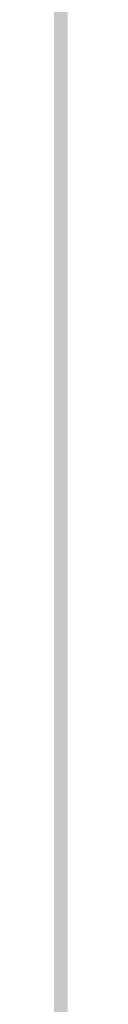
# Model space of a CAD drawing. Units: inches. Extents: x 2083 to 3317, y 1141 to 2115.
# Tile 175 of 256: x 3126.95969 to 3126.95976, y 1263.27402 to 1263.29018. Entities that reach past the tile are written whole.
import ezdxf

# ---------------------------------------------------------------- set-up
doc = ezdxf.new("R2010")
doc.units = ezdxf.units.IN
doc.layers.add('A-ANNO-DIMS', color=2, linetype='Continuous', lineweight=18)
doc.layers.add('A-WALL-PATT', color=251, linetype='Continuous', lineweight=13, true_color=0x636466)
doc.styles.get("Standard").update_dxf_attribs({"font": 'arial.ttf'})
doc.dimstyles.new('ISO-25', dxfattribs={"dimtxt": 12, "dimasz": 12, "dimexe": 1.25, "dimexo": 0.625, "dimtad": 1, "dimlunit": 3, "dimtxsty": 'Standard', "dimcen": 2.5, "dimadec": 0, "dimazin": 0, "dimtfac": 1, "dimtmove": 0, "dimatfit": 3, "dimfxl": 1, "dimarcsym": 0})

# ---------------------------------------------------------------- blocks, each defined once
blk = doc.blocks.new('*D26')
at = {"layer": 'A-ANNO-DIMS', "color": 0, "lineweight": -2, "transparency": 16777216}
for p, q in [((3088.985844, 1274.915092), (3088.985844, 1270.951963)), ((3111.240037, 1274.915092), (3111.240037, 1270.951963)), ((3076.985844, 1272.201963), (2840.262447, 1272.201963)), ((3111.240037, 1272.201963), (3088.985844, 1272.201963)), ((3123.240037, 1272.201963), (3135.240037, 1272.201963))]:
    blk.add_line(p, q, dxfattribs=at)
at = {"layer": 'A-ANNO-DIMS', "color": 0, "transparency": 16777216}
for points in [[(3076.985844, 1274.201963), (3076.985844, 1270.201963), (3088.985844, 1272.201963)], [(3123.240037, 1274.201963), (3123.240037, 1270.201963), (3111.240037, 1272.201963)]]:
    blk.add_solid(points, dxfattribs=at)
at = {"layer": 'Defpoints', "color": 0, "transparency": 16777216}
for p in [(3088.985844, 1275.540092), (3111.240037, 1275.540092), (3088.985844, 1272.201963)]:
    blk.add_point(p, dxfattribs=at)
at = {"layer": 'A-ANNO-DIMS', "color": 0, "transparency": 16777216, "insert": (2952.624146, 1279.031602), "char_height": 12, "attachment_point": 5}
blk.add_mtext('NIGHTSTAND 1\'-10 1/2" TYP.', dxfattribs=at)
blk = doc.blocks.new('*D27')
at = {"layer": 'A-ANNO-DIMS', "color": 0, "lineweight": -2, "transparency": 16777216}
for p, q in [((3114.578165, 1309.794285), (3114.578165, 1321.794285)), ((3111.865037, 1297.794285), (3115.828165, 1297.794285)), ((3114.578165, 1297.794285), (3114.578165, 1275.540092)), ((3111.865037, 1275.540092), (3115.828165, 1275.540092)), ((3114.578165, 1263.540092), (3114.578165, 1140.988591))]:
    blk.add_line(p, q, dxfattribs=at)
at = {"layer": 'A-ANNO-DIMS', "color": 0, "transparency": 16777216}
for points in [[(3112.578165, 1309.794285), (3116.578165, 1309.794285), (3114.578165, 1297.794285)], [(3112.578165, 1263.540092), (3116.578165, 1263.540092), (3114.578165, 1275.540092)]]:
    blk.add_solid(points, dxfattribs=at)
at = {"layer": 'Defpoints', "color": 0, "transparency": 16777216}
for p in [(3111.240037, 1297.794285), (3111.240037, 1275.540092), (3114.578165, 1275.540092)]:
    blk.add_point(p, dxfattribs=at)
at = {"layer": 'A-ANNO-DIMS', "color": 0, "transparency": 16777216, "insert": (3107.748527, 1196.264342), "char_height": 12, "attachment_point": 5, "rotation": 90}
blk.add_mtext('1\'-10 1/2" TYP.', dxfattribs=at)

msp = doc.modelspace()

# ---------------------------------------------------------------- hatches: boundary and pattern name
at = {"layer": 'A-WALL-PATT'}
h = msp.add_hatch(color=256, dxfattribs=at)
h.dxf.hatch_style = 1
h.paths.add_polyline_path([(3126.959783, 2020.76136), (2748.959783, 2020.76136), (2604.959783, 2020.76136), (2226.959783, 2020.76136), (2226.959783, 1702.76136), (2466.959783, 1702.76136), (2466.959783, 1582.76136), (2418.959783, 1582.76136), (2418.959783, 1477.76136), (2226.959783, 1477.76136), (2226.959783, 1263.26136), (2544.959783, 1263.26136), (2544.959783, 1411.76136), (2604.959783, 1411.76136), (2685.959783, 1411.76136), (2685.959783, 1420.76136), (2604.959783, 1420.76136), (2604.959783, 1573.76136), (2604.959783, 1702.76136), (2604.959783, 2011.76136), (2748.959783, 2011.76136), (2748.959783, 1702.76136), (2862.959783, 1702.76136), (2862.959783, 1621.76136), (2871.959783, 1621.76136), (2871.959783, 1702.76136), (2883.959783, 1702.76136), (2883.959783, 1706.939459, -0.026459), (2883.959783, 1711.76136), (2757.959783, 1711.76136), (2757.959783, 1807.76136), (2787.959783, 1807.76136), (2787.959783, 1812.26136), (2757.959783, 1812.26136), (2757.959783, 2011.76136), (2877.959783, 2011.76136), (2877.959783, 1812.26136), (2847.959783, 1812.26136), (2847.959783, 1807.76136), (2889.835742, 1807.76136), (2889.835742, 1812.26136), (2882.459783, 1812.26136), (2882.459783, 2011.76136), (3117.959783, 2011.76136), (3117.959783, 1812.26136), (2937.835742, 1812.26136), (2937.835742, 1807.76136), (2995.709783, 1807.76136), (2995.709783, 1796.117666), (3000.209783, 1796.117666), (3000.209783, 1807.76136), (3117.959783, 1807.76136), (3117.959783, 1711.76136), (3000.209783, 1711.76136), (3000.209783, 1760.117666), (2998.572705, 1760.117666, -0.020711), (2995.709783, 1760.117666), (2995.709783, 1711.76136), (2931.959783, 1711.76136), (2931.959783, 1702.76136), (3126.959783, 1702.76136)])
h.paths.add_polyline_path([(2471.459783, 2011.76136), (2471.459783, 1810.01136), (2462.716936, 1810.01136), (2462.716936, 1805.51136), (2505.959783, 1805.51136), (2505.959783, 1810.01136), (2475.959783, 1810.01136), (2475.959783, 2011.76136), (2595.959783, 2011.76136), (2595.959783, 1810.01136), (2565.959783, 1810.01136), (2565.959783, 1805.51136), (2595.959783, 1805.51136), (2595.959783, 1711.76136), (2235.959783, 1711.76136), (2235.959783, 1805.51136), (2353.709783, 1805.51136), (2353.709783, 1796.054162), (2358.209783, 1796.054162), (2358.209783, 1805.51136), (2414.716936, 1805.51136), (2414.716936, 1810.01136), (2235.959783, 1810.01136), (2235.959783, 2011.76136)], flags=16)
h.paths.add_polyline_path([(2270.204734, 1994.610008), (2270.204734, 1970.610008), (2246.204734, 1970.610008), (2246.204734, 1994.610008)], flags=0)
edge = h.paths.add_edge_path(flags=0)
edge.add_ellipse((2332.027391, 1899.798176), major_axis=(-3.042994, 3.042994), ratio=0.16825245, start_angle=-161.332166, end_angle=-156.307114, ccw=False)
edge.add_ellipse((2333.082037, 1898.74353), major_axis=(-1.054646, 1.054646), ratio=0.4535321, start_angle=-123.371019, end_angle=-94.159107)
edge = h.paths.add_edge_path(flags=0)
edge.add_ellipse((2332.027391, 1968.87629), major_axis=(3.042994, 3.042994), ratio=0.16825245, start_angle=18.667834, end_angle=23.692886)
edge.add_spline(control_points=[(2332.925596, 1970.691105), (2332.226768, 1970.3361), (2330.893709, 1969.658905), (2328.41308, 1970.932138), (2327.203934, 1967.748712), (2324.709596, 1969.955589), (2322.532822, 1967.012354), (2320.012846, 1971.295812), (2317.680308, 1968.157845), (2316.040526, 1967.102047), (2315.426904, 1966.809602)], knot_values=[0, 0, 0, 0, 2.267059, 4.324559, 6.685584, 8.878641, 11.121502, 14.300359, 17.755284, 19.732645, 19.732645, 19.732645, 19.732645], degree=3, periodic=0)
edge.add_ellipse((2332.027391, 1968.87629), major_axis=(3.042994, 3.042994), ratio=0.16825245, start_angle=18.667834, end_angle=23.692886, ccw=False)
edge.add_ellipse((2333.082037, 1969.930936), major_axis=(1.054646, 1.054646), ratio=0.4535321, start_angle=56.628981, end_angle=85.840893, ccw=False)
edge = h.paths.add_edge_path(flags=0)
edge.add_spline(control_points=[(2296.428287, 1967.987908), (2293.627804, 1965.336314), (2287.703624, 1959.727094), (2299.74386, 1949.995699), (2294.532591, 1935.668528), (2290.573228, 1920.603512), (2293.394124, 1909.973691), (2296.185407, 1904.966543)], knot_values=[0.099185, 0.099185, 0.099185, 0.099185, 0.345301, 0.619822, 0.982653, 1.386093, 1.810555, 1.810555, 1.810555, 1.810555], degree=3, periodic=0)
edge.add_spline(control_points=[(2296.185407, 1904.966543), (2297.383582, 1902.6193), (2298.000969, 1901.949312), (2298.55297, 1901.468155)], knot_values=[0.006246, 0.006246, 0.006246, 0.006246, 0.055476, 0.055476, 0.055476, 0.055476], degree=3, periodic=0)
edge.add_spline(control_points=[(2298.55297, 1901.468155), (2297.258612, 1900.923224), (2295.225294, 1900.232126), (2293.060229, 1900.614205), (2292.101423, 1900.788415), (2292.089578, 1900.790568)], knot_values=[0.312835, 0.312835, 0.312835, 0.312835, 0.40178, 0.474987, 0.475903, 0.475903, 0.475903, 0.475903], degree=3, periodic=0)
edge.add_arc((2292.793646, 1904.664109), 3.937008, 215.420897, 259.698179, ccw=False)
edge.add_spline(control_points=[(2289.585314, 1902.382304), (2289.476652, 1902.535087), (2289.36848, 1902.688035), (2289.260865, 1902.84117)], knot_values=[0.102872, 0.102872, 0.102872, 0.102872, 0.116896, 0.116896, 0.116896, 0.116896], degree=3, periodic=0)
edge.add_spline(control_points=[(2289.260865, 1902.84117), (2288.686604, 1902.550192), (2287.640048, 1902.019902), (2285.881337, 1901.873954), (2283.852972, 1901.504352), (2281.719987, 1899.710538), (2278.466991, 1899.492942), (2276.157136, 1901.883202), (2272.258953, 1899.804071), (2267.777605, 1901.843183), (2262.243882, 1900.184033), (2257.414927, 1901.782061), (2254.318374, 1900.72612), (2253.178285, 1900.337343)], knot_values=[0, 0, 0, 0, 1.907977, 3.477176, 5.261074, 7.972851, 11.680248, 13.717921, 16.939592, 22.789562, 27.502503, 33.595215, 37.145618, 37.145618, 37.145618, 37.145618], degree=3, periodic=0)
edge.add_line((2253.178285, 1900.337343), (2250.24424, 1902.84117))
edge.add_line((2250.24424, 1902.84117), (2250.24424, 1965.833296))
edge.add_line((2250.24424, 1965.833296), (2253.178285, 1968.337123))
edge.add_spline(control_points=[(2253.178285, 1968.337123), (2254.318374, 1967.948346), (2257.414927, 1966.892405), (2262.243882, 1968.490433), (2267.777605, 1966.831283), (2271.52673, 1968.537217), (2273.875914, 1967.828289), (2274.206701, 1967.727642)], knot_values=[0, 0, 0, 0, 0.09018, 0.244935, 0.364644, 0.513233, 0.537855, 0.537855, 0.537855, 0.537855], degree=3, periodic=0)
edge.add_arc((2274.352887, 1963.793349), 3.937008, 72.051134, 92.127949, ccw=False)
edge.add_arc((2281.296933, 1985.230003), 18.596298, 252.0511336, 288.5657217)
edge.add_arc((2292.316717, 1956.02888), 12.646081, 71.0267879, 113.7782184, ccw=False)
edge = h.paths.add_edge_path(flags=0)
edge.add_spline(control_points=[(2274.899415, 1951.856195), (2275.066156, 1951.616592), (2275.232687, 1951.376588), (2275.397987, 1951.135855)], knot_values=[1.409916, 1.409916, 1.409916, 1.409916, 1.43159, 1.43159, 1.43159, 1.43159], degree=3, periodic=0)
edge.add_spline(control_points=[(2275.397987, 1951.135855), (2275.792106, 1950.561885), (2276.179231, 1949.983774), (2276.545546, 1949.397103)], knot_values=[1.358238, 1.358238, 1.358238, 1.358238, 1.409916, 1.409916, 1.409916, 1.409916], degree=3, periodic=0)
edge.add_line((2276.545546, 1949.397103), (2277.437289, 1947.862185))
edge.add_spline(control_points=[(2277.437289, 1947.862185), (2276.303834, 1945.673115), (2274.639698, 1942.426882), (2274.631615, 1938.0939), (2272.799124, 1930.85155), (2274.356426, 1943.897046), (2275.947681, 1947.923356), (2276.545546, 1949.397103)], knot_values=[0.005632, 0.005632, 0.005632, 0.005632, 0.186014, 0.266002, 0.357087, 0.59639, 0.739732, 0.739732, 0.739732, 0.739732], degree=3, periodic=0)
edge.add_spline(control_points=[(2276.545546, 1949.397103), (2276.179231, 1949.983774), (2275.792106, 1950.561885), (2275.397987, 1951.135855)], knot_values=[1.358238, 1.358238, 1.358238, 1.358238, 1.409916, 1.409916, 1.409916, 1.409916], degree=3, periodic=0)
edge.add_spline(control_points=[(2275.397987, 1951.135855), (2274.9425, 1950.080452), (2274.20776, 1948.025272), (2273.934602, 1944.851477), (2272.468534, 1937.627489), (2273.466216, 1945.696466), (2274.700615, 1951.059472), (2274.899415, 1951.856195)], knot_values=[0.104364, 0.104364, 0.104364, 0.104364, 0.189636, 0.269624, 0.36071, 0.600013, 0.644622, 0.644622, 0.644622, 0.644622], degree=3, periodic=0)
h.paths.add_polyline_path([(2269.167514, 1963.127573, -0.357527), (2268.170633, 1960.97637, -0.092561), (2268.170633, 1939.436325, -0.357527), (2269.167514, 1937.285122, -0.357527), (2267.01631, 1938.282002, -0.164785), (2254.685581, 1938.282002, -0.357527), (2252.534378, 1937.285122, -0.357527), (2253.531259, 1939.436325, -0.092561), (2253.531259, 1960.97637, -0.357527), (2252.534378, 1963.127573, -0.357527), (2254.685581, 1962.130692, -0.164785), (2267.01631, 1962.130692, -0.357527)], flags=0)
h.paths.add_polyline_path([(2248.874068, 1967.8018), (2248.874068, 1957.02771), (2249.457783, 1957.02771), (2249.457783, 1911.646756), (2248.874068, 1911.646756), (2248.874068, 1900.872666), (2246.511863, 1900.872666, 0.197327), (2244.149658, 1902.456873), (2244.149658, 1966.217592, 0.197327), (2246.511863, 1967.8018)], flags=0)
h.paths.add_polyline_path([(2269.167514, 1931.389344, -0.357527), (2268.170633, 1929.238141, -0.092561), (2268.170633, 1907.698096, -0.357527), (2269.167514, 1905.546893, -0.357527), (2267.01631, 1906.543774, -0.164785), (2254.685581, 1906.543774, -0.357527), (2252.534378, 1905.546893, -0.357527), (2253.531259, 1907.698096, -0.092561), (2253.531259, 1929.238141, -0.357527), (2252.534378, 1931.389344, -0.357527), (2254.685581, 1930.392463, -0.164785), (2267.01631, 1930.392463, -0.357527)], flags=0)
edge = h.paths.add_edge_path(flags=0)
edge.add_spline(control_points=[(2276.196858, 1906.723702), (2276.168144, 1909.028928), (2276.114049, 1913.371852), (2270.598417, 1924.924978), (2273.905175, 1919.012779), (2275.921711, 1916.262063), (2275.47457, 1912.402149), (2277.257874, 1910.380621), (2276.696044, 1908.225036), (2276.646218, 1906.813023), (2276.617825, 1906.008407)], knot_values=[0, 0, 0, 0, 8.61026, 16.221274, 18.843057, 23.804898, 27.440828, 29.356102, 31.203478, 33.650687, 33.650687, 33.650687, 33.650687], degree=3, periodic=0)
edge.add_spline(control_points=[(2276.617825, 1906.008407), (2276.623313, 1905.624144), (2276.497738, 1904.628661), (2275.441779, 1903.854725), (2274.937314, 1903.08045), (2274.85908, 1902.84117)], knot_values=[0.156488, 0.156488, 0.156488, 0.156488, 0.184398, 0.231376, 0.250598, 0.250598, 0.250598, 0.250598], degree=3, periodic=0)
edge.add_line((2274.85908, 1902.84117), (2276.50598, 1902.84117))
edge.add_spline(control_points=[(2276.50598, 1902.84117), (2276.788308, 1903.08494), (2277.665071, 1904.125196), (2278.249538, 1904.340738), (2277.653872, 1908.527387), (2278.15567, 1906.227808), (2278.100464, 1905.285948), (2278.846675, 1904.069005), (2277.856785, 1903.414948), (2277.874191, 1902.99105), (2277.903562, 1902.84117)], knot_values=[0.059574, 0.059574, 0.059574, 0.059574, 0.080753, 0.103741, 0.16972, 0.176036, 0.207137, 0.240474, 0.262341, 0.27366, 0.27366, 0.27366, 0.27366], degree=3, periodic=0)
edge.add_line((2277.903562, 1902.84117), (2280.029825, 1902.84117))
edge.add_spline(control_points=[(2280.029825, 1902.84117), (2279.888221, 1903.088398), (2279.499257, 1903.981551), (2280.152284, 1905.939349), (2278.103615, 1909.657757), (2279.762395, 1907.185285), (2280.3279, 1904.874861), (2280.485109, 1903.48959), (2281.463269, 1903.249432), (2281.758343, 1902.936497), (2281.834036, 1902.84117)], knot_values=[0.013856, 0.013856, 0.013856, 0.013856, 0.034874, 0.088867, 0.107879, 0.126738, 0.158714, 0.193757, 0.217487, 0.226722, 0.226722, 0.226722, 0.226722], degree=3, periodic=0)
edge.add_spline(control_points=[(2281.834036, 1902.84117), (2281.787535, 1902.826703), (2281.647022, 1902.782988), (2281.395527, 1902.85949), (2281.088077, 1902.985242), (2280.720683, 1903.060902), (2280.333451, 1903.025726), (2280.124767, 1902.898879), (2280.029825, 1902.84117)], knot_values=[0, 0, 0, 0, 0.14413, 0.435517, 0.749276, 1.153046, 1.548371, 1.878348, 1.878348, 1.878348, 1.878348], degree=3, periodic=0)
edge.add_line((2280.029825, 1902.84117), (2277.903562, 1902.84117))
edge.add_spline(control_points=[(2277.903562, 1902.84117), (2277.892855, 1902.795855), (2277.865396, 1902.679637), (2277.607479, 1902.687483), (2277.27405, 1902.8007), (2276.837921, 1902.619775), (2276.583807, 1902.789261), (2276.50598, 1902.84117)], knot_values=[0, 0, 0, 0, 0.127189, 0.326199, 0.628009, 1.24357, 1.515331, 1.515331, 1.515331, 1.515331], degree=3, periodic=0)
edge.add_line((2276.50598, 1902.84117), (2274.85908, 1902.84117))
edge.add_spline(control_points=[(2274.85908, 1902.84117), (2274.814437, 1902.898587), (2274.72513, 1903.013446), (2274.493477, 1903.118968), (2274.244285, 1902.960539), (2273.937121, 1903.184942), (2273.614039, 1902.983143), (2273.408316, 1902.883045), (2273.322254, 1902.84117)], knot_values=[0, 0, 0, 0, 0.21843, 0.436957, 0.687977, 0.990379, 1.398396, 1.69185, 1.69185, 1.69185, 1.69185], degree=3, periodic=0)
edge.add_spline(control_points=[(2273.322254, 1902.84117), (2273.61674, 1903.445692), (2274.273998, 1904.538253), (2276.027239, 1904.573702), (2276.206963, 1906.583637), (2276.196858, 1906.723702)], knot_values=[0.012227, 0.012227, 0.012227, 0.012227, 0.059472, 0.106218, 0.134458, 0.134458, 0.134458, 0.134458], degree=3, periodic=0)
h.paths.add_polyline_path([(2270.776054, 1897.789828), (2270.776054, 1873.789828), (2246.776054, 1873.789828), (2246.776054, 1897.789828)], flags=0)
h.paths.add_polyline_path([(2353.709783, 1760.005059), (2353.709783, 1760.054162), (2358.209783, 1760.054162, -0.033729)], flags=0)
h.paths.add_polyline_path([(2321.819119, 1737.529186), (2341.995327, 1737.529186, -0.414214), (2343.203273, 1736.321241), (2343.203273, 1721.020596, -0.414214), (2341.995327, 1719.812651), (2321.819119, 1719.812651, -0.414214), (2320.611173, 1721.020596), (2320.611173, 1736.321241, -0.414214)], flags=0)
h.paths.add_polyline_path([(2324.23501, 1736.321241), (2339.579436, 1736.321241, -0.414214), (2341.995327, 1733.905349), (2341.995327, 1725.44973, -0.414214), (2339.579436, 1723.033839), (2333.680588, 1723.033839), (2333.845317, 1722.045467, -0.870646), (2335.425399, 1721.825893, -0.767327), (2333.922694, 1721.423245), (2331.291024, 1721.423245, -0.767327), (2329.788319, 1721.825893, -0.870646), (2331.368401, 1722.045467), (2331.53313, 1723.033839), (2324.23501, 1723.033839, -0.414214), (2321.819119, 1725.44973), (2321.819119, 1733.905349, -0.414214)], flags=0)
h.paths.add_polyline_path([(2570.483789, 1928.615444), (2589.683789, 1928.615444), (2590.168829, 1928.615444), (2590.168829, 1904.993397), (2570.483789, 1904.993397)], flags=0)
h.paths.add_polyline_path([(2574.447324, 1927.263822, -1), (2572.828836, 1927.263822, -1)], flags=0)
h.paths.add_polyline_path([(2573.089867, 1926.940877), (2573.925032, 1927.776042), (2574.147743, 1927.553332), (2573.312577, 1926.718166)], flags=0)
h.paths.add_polyline_path([(2578.779065, 1919.729618, -1), (2571.591663, 1919.729618, -1)], flags=0)
h.paths.add_polyline_path([(2578.385364, 1919.729618, -1), (2571.985364, 1919.729618, -1)], flags=0)
h.paths.add_polyline_path([(2331.595764, 1729.476216, -1), (2333.617954, 1729.476216, -1)], flags=0)
h.paths.add_polyline_path([(2578.034228, 1927.263822, -1), (2576.41574, 1927.263822, -1)], flags=0)
h.paths.add_polyline_path([(2576.688851, 1927.531089), (2576.911562, 1927.753799), (2577.746728, 1926.918634), (2577.524017, 1926.695923)], flags=0)
h.paths.add_polyline_path([(2578.139065, 1909.859539, -1), (2572.231663, 1909.859539, -1)], flags=0)
h.paths.add_polyline_path([(2577.745364, 1909.859539, -1), (2572.625364, 1909.859539, -1)], flags=0)
h.paths.add_polyline_path([(2583.797718, 1927.263822, -1), (2582.179229, 1927.263822, -1)], flags=0)
h.paths.add_polyline_path([(2582.718649, 1927.753799), (2583.553814, 1926.918634), (2583.331103, 1926.695923), (2582.495938, 1927.531089)], flags=0)
h.paths.add_polyline_path([(2582.495938, 1927.531089), (2582.718649, 1927.753799), (2583.553814, 1926.918634), (2583.331103, 1926.695923)], flags=0)
h.paths.add_polyline_path([(2587.739065, 1920.529618, -1), (2581.831663, 1920.529618, -1)], flags=0)
h.paths.add_polyline_path([(2587.345364, 1920.529618, -1), (2582.225364, 1920.529618, -1)], flags=0)
h.paths.add_polyline_path([(2587.384622, 1927.263822, -1), (2585.766133, 1927.263822, -1)], flags=0)
h.paths.add_polyline_path([(2586.081993, 1926.980247), (2586.917158, 1927.815412), (2587.139869, 1927.592702), (2586.304703, 1926.757536)], flags=0)
h.paths.add_polyline_path([(2588.379065, 1910.659539, -1), (2581.191663, 1910.659539, -1)], flags=0)
h.paths.add_polyline_path([(2587.985364, 1910.659539, -1), (2581.585364, 1910.659539, -1)], flags=0)
h.paths.add_polyline_path([(2417.167729, 1729.477895), (2437.343937, 1729.477895, -0.414214), (2438.551883, 1728.26995), (2438.551883, 1712.969306, -0.414214), (2437.343937, 1711.76136), (2417.167729, 1711.76136, -0.414214), (2415.959783, 1712.969306), (2415.959783, 1728.26995, -0.414214)], flags=0)
h.paths.add_polyline_path([(2419.58362, 1728.26995), (2434.928046, 1728.26995, -0.414214), (2437.343937, 1725.854059), (2437.343937, 1717.39844, -0.414214), (2434.928046, 1714.982548), (2429.029199, 1714.982548), (2429.193927, 1713.994176, -0.870646), (2430.774009, 1713.774603, -0.767327), (2429.271304, 1713.371954), (2426.639634, 1713.371954, -0.767327), (2425.136929, 1713.774603, -0.870646), (2426.717011, 1713.994176), (2426.88174, 1714.982548), (2419.58362, 1714.982548, -0.414214), (2417.167729, 1717.39844), (2417.167729, 1725.854059, -0.414214)], flags=0)
h.paths.add_polyline_path([(2419.58362, 1728.26995), (2434.928046, 1728.26995, -0.414214), (2437.343937, 1725.854059), (2437.343937, 1717.39844, -0.414214), (2434.928046, 1714.982548), (2429.029199, 1714.982548), (2428.358118, 1719.009034), (2427.552821, 1719.009034), (2426.88174, 1714.982548), (2419.58362, 1714.982548, -0.414214), (2417.167729, 1717.39844), (2417.167729, 1725.854059, -0.414214)], flags=0)
h.paths.add_polyline_path([(2426.944374, 1721.424925, -1), (2428.966564, 1721.424925, -1)], flags=0)
h.paths.add_polyline_path([(2475.959783, 1702.76136), (2595.959783, 1702.76136), (2595.959783, 1582.76136), (2475.959783, 1582.76136)], flags=16)
h.paths.add_polyline_path([(2427.959783, 1573.76136), (2595.959783, 1573.76136), (2595.959783, 1468.76136), (2595.959783, 1420.76136), (2384.459783, 1420.76136), (2384.459783, 1468.76136), (2427.959783, 1468.76136)], flags=16)
h.paths.add_polyline_path([(2379.959783, 1468.76136), (2379.959783, 1420.76136), (2235.959783, 1420.76136), (2235.959783, 1468.76136)], flags=16)
h.paths.add_polyline_path([(2317.815996, 1466.695767), (2337.992205, 1466.695767, -0.414214), (2339.20015, 1465.487821), (2339.20015, 1450.187177, -0.414214), (2337.992205, 1448.979232), (2317.815996, 1448.979232, -0.414214), (2316.608051, 1450.187177), (2316.608051, 1465.487821, -0.414214)], flags=0)
h.paths.add_polyline_path([(2320.231887, 1465.487821), (2335.576313, 1465.487821, -0.414214), (2337.992205, 1463.07193), (2337.992205, 1454.616311, -0.414214), (2335.576313, 1452.20042), (2329.677466, 1452.20042), (2329.842195, 1451.212047, -0.870646), (2331.422276, 1450.992474, -0.767327), (2329.919571, 1450.589826), (2327.287902, 1450.589826, -0.767327), (2325.785197, 1450.992474, -0.870646), (2327.365278, 1451.212047), (2327.530007, 1452.20042), (2320.231887, 1452.20042, -0.414214), (2317.815996, 1454.616311), (2317.815996, 1463.07193, -0.414214)], flags=0)
h.paths.add_polyline_path([(2320.231887, 1465.487821), (2335.576313, 1465.487821, -0.414214), (2337.992205, 1463.07193), (2337.992205, 1454.616311, -0.414214), (2335.576313, 1452.20042), (2329.677466, 1452.20042), (2329.006385, 1456.226905), (2328.201088, 1456.226905), (2327.530007, 1452.20042), (2320.231887, 1452.20042, -0.414214), (2317.815996, 1454.616311), (2317.815996, 1463.07193, -0.414214)], flags=0)
h.paths.add_polyline_path([(2327.592641, 1458.642796, -1), (2329.614832, 1458.642796, -1)], flags=0)
h.paths.add_polyline_path([(2244.411744, 1433.340453), (2241.920945, 1433.340453, -0.414214), (2240.017856, 1435.243542), (2240.017856, 1440.952808, -0.414211), (2241.920925, 1442.855897), (2244.411744, 1442.855897, -1.976472)], flags=0)
h.paths.add_polyline_path([(2245.356888, 1434.397536, -0.414214), (2245.356888, 1441.798814, -2.144098)], flags=0)
h.paths.add_polyline_path([(2535.959783, 1416.26136), (2535.959783, 1272.26136), (2235.959783, 1272.26136), (2235.959783, 1416.26136)], flags=16)
h.paths.add_polyline_path([(2260.119561, 1384.292841), (2260.119561, 1362.038649), (2237.865369, 1362.038649), (2237.865369, 1384.292841)], flags=0)
edge = h.paths.add_edge_path(flags=0)
edge.add_line((2318.251847, 1362.093298), (2318.145797, 1362.000973))
edge.add_ellipse((2317.445116, 1360.431044), major_axis=(2.82164, 2.82164), ratio=0.16825245, start_angle=18.667834, end_angle=20.948127, ccw=False)
edge.add_ellipse((2318.423045, 1361.408974), major_axis=(0.977929, 0.977929), ratio=0.4535321, start_angle=56.628981, end_angle=70.226201, ccw=False)
edge = h.paths.add_edge_path(flags=0)
edge.add_line((2319.10737, 1295.571078), (2319.015044, 1295.677128))
edge.add_ellipse((2317.445116, 1296.377809), major_axis=(-2.82164, 2.82164), ratio=0.16825245, start_angle=-161.332166, end_angle=-159.051873, ccw=False)
edge.add_ellipse((2318.423045, 1295.39988), major_axis=(-0.977929, 0.977929), ratio=0.4535321, start_angle=-123.371019, end_angle=-109.773799)
edge = h.paths.add_edge_path(flags=0)
edge.add_spline(control_points=[(2284.210349, 1301.170219), (2284.580688, 1300.444719), (2284.891189, 1299.892024), (2285.159553, 1299.461018)], knot_values=[0.039066, 0.039066, 0.039066, 0.039066, 0.055476, 0.055476, 0.055476, 0.055476], degree=3, periodic=0)
edge.add_line((2285.159553, 1299.461018), (2284.210349, 1301.170219))
edge = h.paths.add_edge_path(flags=0)
edge.add_line((2280.412458, 1297.298013), (2283.369991, 1297.036122))
edge.add_line((2283.369991, 1297.036122), (2286.40569, 1297.92631))
edge.add_spline(control_points=[(2286.40569, 1297.92631), (2285.305487, 1297.463119), (2284.344777, 1297.129151), (2283.369991, 1297.036122)], knot_values=[0.394369, 0.394369, 0.394369, 0.394369, 0.475903, 0.475903, 0.475903, 0.475903], degree=3, periodic=0)
edge.add_spline(control_points=[(2283.369991, 1297.036122), (2283.28139, 1297.027666), (2282.316289, 1296.957336), (2281.312502, 1297.134479), (2280.423441, 1297.296016), (2280.412458, 1297.298013)], knot_values=[0.312835, 0.312835, 0.312835, 0.312835, 0.320246, 0.393453, 0.394369, 0.394369, 0.394369, 0.394369], degree=3, periodic=0)
edge = h.paths.add_edge_path(flags=0)
edge.add_line((2284.435561, 1359.607285), (2280.446291, 1355.328047))
edge.add_line((2280.446291, 1355.328047), (2279.579987, 1351.017754))
edge.add_line((2279.579987, 1351.017754), (2282.412974, 1346.580433))
edge.add_spline(control_points=[(2282.412974, 1346.580433), (2283.153331, 1345.589236), (2284.252896, 1344.028897), (2284.801037, 1342.387167), (2284.935162, 1341.805544)], knot_values=[1.240098, 1.240098, 1.240098, 1.240098, 1.332892, 1.382712, 1.382712, 1.382712, 1.382712], degree=3, periodic=0)
edge.add_spline(control_points=[(2284.935162, 1341.805544), (2285.319108, 1340.1406), (2285.233029, 1338.409204), (2284.909938, 1336.654122)], knot_values=[1.097484, 1.097484, 1.097484, 1.097484, 1.240098, 1.240098, 1.240098, 1.240098], degree=3, periodic=0)
edge.add_spline(control_points=[(2284.909938, 1336.654122), (2284.586848, 1334.89904), (2284.026745, 1333.120272), (2283.462644, 1331.360585)], knot_values=[0.95487, 0.95487, 0.95487, 0.95487, 1.097484, 1.097484, 1.097484, 1.097484], degree=3, periodic=0)
edge.add_line((2283.462644, 1331.360585), (2281.890376, 1326.153357))
edge.add_line((2281.890376, 1326.153357), (2280.756259, 1321.056089))
edge.add_line((2280.756259, 1321.056089), (2280.299205, 1316.001977))
edge.add_line((2280.299205, 1316.001977), (2280.715933, 1310.950068))
edge.add_line((2280.715933, 1310.950068), (2282.028094, 1305.972137))
edge.add_line((2282.028094, 1305.972137), (2284.210349, 1301.170219))
edge.add_spline(control_points=[(2284.210349, 1301.170219), (2283.340731, 1302.730185), (2282.611904, 1304.336493), (2282.028094, 1305.972137)], knot_values=[0.099185, 0.099185, 0.099185, 0.099185, 0.241799, 0.241799, 0.241799, 0.241799], degree=3, periodic=0)
edge.add_spline(control_points=[(2282.028094, 1305.972137), (2281.444283, 1307.60778), (2281.005489, 1309.272759), (2280.715933, 1310.950068)], knot_values=[0.241799, 0.241799, 0.241799, 0.241799, 0.384413, 0.384413, 0.384413, 0.384413], degree=3, periodic=0)
edge.add_spline(control_points=[(2280.715933, 1310.950068), (2280.433241, 1312.587613), (2280.289386, 1314.276959), (2280.298894, 1315.962032), (2280.299205, 1316.001977)], knot_values=[0.384413, 0.384413, 0.384413, 0.384413, 0.523647, 0.527028, 0.527028, 0.527028, 0.527028], degree=3, periodic=0)
edge.add_spline(control_points=[(2280.299205, 1316.001977), (2280.312326, 1317.686955), (2280.477871, 1319.367926), (2280.756259, 1321.056089)], knot_values=[0.527028, 0.527028, 0.527028, 0.527028, 0.669642, 0.669642, 0.669642, 0.669642], degree=3, periodic=0)
edge.add_spline(control_points=[(2280.756259, 1321.056089), (2281.034648, 1322.744252), (2281.42588, 1324.439608), (2281.890376, 1326.153357)], knot_values=[0.669642, 0.669642, 0.669642, 0.669642, 0.812256, 0.812256, 0.812256, 0.812256], degree=3, periodic=0)
edge.add_spline(control_points=[(2281.890376, 1326.153357), (2282.264383, 1327.533251), (2282.78787, 1329.26181), (2283.352751, 1331.01778), (2283.462644, 1331.360585)], knot_values=[0.812256, 0.812256, 0.812256, 0.812256, 0.927087, 0.95487, 0.95487, 0.95487, 0.95487], degree=3, periodic=0)
edge.add_line((2283.462644, 1331.360585), (2284.909938, 1336.654122))
edge.add_line((2284.909938, 1336.654122), (2284.935162, 1341.805544))
edge.add_line((2284.935162, 1341.805544), (2282.412974, 1346.580433))
edge.add_spline(control_points=[(2282.412974, 1346.580433), (2281.275127, 1348.103792), (2280.078447, 1349.570318), (2279.579987, 1351.017754)], knot_values=[1.382712, 1.382712, 1.382712, 1.382712, 1.525326, 1.525326, 1.525326, 1.525326], degree=3, periodic=0)
edge.add_spline(control_points=[(2279.579987, 1351.017754), (2279.443282, 1351.414721), (2279.136312, 1352.856922), (2279.73519, 1354.290385), (2280.446291, 1355.328047)], knot_values=[1.525326, 1.525326, 1.525326, 1.525326, 1.564439, 1.667941, 1.667941, 1.667941, 1.667941], degree=3, periodic=0)
edge.add_spline(control_points=[(2280.446291, 1355.328047), (2281.426113, 1356.757835), (2282.930837, 1358.18256), (2284.435561, 1359.607285)], knot_values=[1.667941, 1.667941, 1.667941, 1.667941, 1.810555, 1.810555, 1.810555, 1.810555], degree=3, periodic=0)
edge.add_arc((2280.623075, 1348.518181), 11.72618, 71.0267879, 113.7782184)
edge.add_arc((2270.404892, 1375.595156), 17.243567, 252.0511336, 288.5657217, ccw=False)
edge.add_arc((2263.965969, 1355.717847), 3.650622, 72.051134, 92.127949)
edge.add_arc((2263.965969, 1355.717847), 3.650622, 92.127949, 177.98513)
edge.add_spline(control_points=[(2260.317604, 1355.846199), (2260.260417, 1354.220668), (2260.551278, 1350.186547), (2262.999344, 1346.766251), (2264.472741, 1344.649024)], knot_values=[1.43159, 1.43159, 1.43159, 1.43159, 1.564144, 1.770695, 1.770695, 1.770695, 1.770695], degree=3, periodic=0)
edge.add_line((2264.472741, 1344.649024), (2264.93559, 1343.98253))
edge.add_spline(control_points=[(2263.801044, 1340.248105), (2263.843238, 1340.514088), (2264.067244, 1341.756465), (2264.512693, 1343.002453), (2264.935047, 1343.981083)], knot_values=[0.53657, 0.53657, 0.53657, 0.53657, 0.559349, 0.644622, 0.644622, 0.644622, 0.644622], degree=3, periodic=0)
edge.add_spline(control_points=[(2264.935047, 1343.981083), (2265.117771, 1343.714975), (2265.298875, 1343.447906), (2265.476756, 1343.179365)], knot_values=[1.384077, 1.384077, 1.384077, 1.384077, 1.409916, 1.409916, 1.409916, 1.409916], degree=3, periodic=0)
edge.add_spline(control_points=[(2265.476756, 1343.179365), (2265.654637, 1342.910823), (2265.829296, 1342.64081), (2265.99913, 1342.368812)], knot_values=[1.358238, 1.358238, 1.358238, 1.358238, 1.384077, 1.384077, 1.384077, 1.384077], degree=3, periodic=0)
edge.add_line((2265.99913, 1342.368812), (2266.826006, 1340.945547))
edge.add_spline(control_points=[(2266.826006, 1340.945547), (2268.894401, 1337.089691), (2271.398173, 1325.843001), (2270.516164, 1310.568557), (2275.919376, 1301.860609), (2277.789511, 1299.19945)], knot_values=[0.116896, 0.116896, 0.116896, 0.116896, 0.472987, 1.050969, 1.313793, 1.313793, 1.313793, 1.313793], degree=3, periodic=0)
edge.add_spline(control_points=[(2277.789511, 1299.19945), (2277.839405, 1299.128452), (2277.889428, 1299.057498), (2277.939572, 1298.986584)], knot_values=[0.109884, 0.109884, 0.109884, 0.109884, 0.116896, 0.116896, 0.116896, 0.116896], degree=3, periodic=0)
edge.add_line((2277.939572, 1298.986584), (2277.788849, 1299.199114))
edge.add_spline(control_points=[(2277.788849, 1299.199114), (2277.256582, 1298.929414), (2276.28635, 1298.437902), (2275.039352, 1298.334419), (2274.38333, 1298.238895), (2274.215254, 1298.209338)], knot_values=[33.12187, 33.12187, 33.12187, 33.12187, 35.029056, 36.598255, 37.144827, 37.144827, 37.144827, 37.144827], degree=3, periodic=0)
edge.add_line((2274.215254, 1298.209338), (2273.073147, 1297.892961))
edge.add_spline(control_points=[(2273.073147, 1297.892961), (2272.322936, 1297.579784), (2271.039151, 1296.510508), (2269.248395, 1296.226062), (2268.4231, 1296.374654)], knot_values=[26.532584, 26.532584, 26.532584, 26.532584, 29.198919, 31.839101, 31.839101, 31.839101, 31.839101], degree=3, periodic=0)
edge.add_line((2268.4231, 1296.374654), (2263.878501, 1297.457534))
edge.add_spline(control_points=[(2263.878501, 1297.457534), (2263.556077, 1297.359435), (2261.860306, 1296.838694), (2260.23878, 1297.282407), (2258.933454, 1297.516461)], knot_values=[15.919551, 15.919551, 15.919551, 15.919551, 16.939592, 21.226067, 21.226067, 21.226067, 21.226067], degree=3, periodic=0)
edge.add_line((2258.933454, 1297.516461), (2254.055233, 1297.32901))
edge.add_spline(control_points=[(2254.055233, 1297.32901), (2253.755525, 1297.295815), (2252.113683, 1297.165174), (2250.461869, 1297.544221), (2249.129686, 1297.667882)], knot_values=[5.306517, 5.306517, 5.306517, 5.306517, 6.276435, 10.613034, 10.613034, 10.613034, 10.613034], degree=3, periodic=0)
edge.add_line((2249.129686, 1297.667882), (2244.33165, 1296.877756))
edge.add_line((2244.33165, 1296.877756), (2241.611033, 1299.19945))
edge.add_line((2241.611033, 1299.19945), (2241.611033, 1357.609404))
edge.add_line((2241.611033, 1357.609404), (2244.33165, 1359.931097))
edge.add_line((2244.33165, 1359.931097), (2252.728823, 1359.542692))
edge.add_spline(control_points=[(2252.728823, 1359.542692), (2252.870939, 1359.54644), (2253.30574, 1359.548172), (2253.739845, 1359.514274), (2254.031742, 1359.482426)], knot_values=[0.233291, 0.233291, 0.233291, 0.233291, 0.244935, 0.268927, 0.268927, 0.268927, 0.268927], degree=3, periodic=0)
edge.add_line((2254.031742, 1359.482426), (2259.58719, 1359.41639))
edge.add_spline(control_points=[(2259.58719, 1359.41639), (2260.677068, 1359.628503), (2262.073197, 1359.897003), (2263.523692, 1359.459278), (2263.830417, 1359.365952)], knot_values=[0.422516, 0.422516, 0.422516, 0.422516, 0.513233, 0.537855, 0.537855, 0.537855, 0.537855], degree=3, periodic=0)
edge.add_arc((2263.965969, 1355.717847), 3.650622, 72.051134, 92.127949, ccw=False)
edge.add_arc((2270.404892, 1375.595156), 17.243567, 252.0511336, 288.5657217)
edge.add_arc((2280.623075, 1348.518181), 11.72618, 71.0267879, 113.7782184, ccw=False)
h.paths.add_polyline_path([(2240.34053, 1359.434715), (2240.34053, 1349.444353), (2240.881785, 1349.444353), (2240.881785, 1307.3645), (2240.34053, 1307.3645), (2240.34053, 1297.374138), (2238.150157, 1297.374138, 0.197327), (2235.959783, 1298.843108), (2235.959783, 1357.965746, 0.197327), (2238.150157, 1359.434715)], flags=0)
h.paths.add_polyline_path([(2259.15779, 1355.1005, -0.357527), (2258.233425, 1353.10578, -0.092561), (2258.233425, 1333.132601, -0.357527), (2259.15779, 1331.13788, -0.357527), (2257.16307, 1332.062246, -0.164785), (2245.729302, 1332.062246, -0.357527), (2243.734582, 1331.13788, -0.357527), (2244.658947, 1333.132601, -0.092561), (2244.658947, 1353.10578, -0.357527), (2243.734582, 1355.1005, -0.357527), (2245.729302, 1354.176135, -0.164785), (2257.16307, 1354.176135, -0.357527)], flags=0)
edge = h.paths.add_edge_path(flags=0)
edge.add_line((2265.99913, 1342.368812), (2266.826006, 1340.945547))
edge.add_line((2266.826006, 1340.945547), (2265.307557, 1337.814066))
edge.add_line((2265.307557, 1337.814066), (2264.358232, 1334.652939))
edge.add_line((2264.358232, 1334.652939), (2264.262012, 1333.799705))
edge.add_spline(control_points=[(2264.262012, 1333.799705), (2264.208357, 1333.187055), (2264.16206, 1332.365525), (2264.007144, 1331.413933), (2263.969049, 1331.201834)], knot_values=[0.464444, 0.464444, 0.464444, 0.464444, 0.516691, 0.531608, 0.531608, 0.531608, 0.531608], degree=3, periodic=0)
edge.add_spline(control_points=[(2263.969049, 1331.201834), (2263.774535, 1330.118873), (2263.42437, 1328.790839), (2263.25742, 1328.530652), (2263.234028, 1328.514612)], knot_values=[0.372682, 0.372682, 0.372682, 0.372682, 0.44885, 0.464444, 0.464444, 0.464444, 0.464444], degree=3, periodic=0)
edge.add_spline(control_points=[(2263.234028, 1328.514612), (2263.096382, 1328.420227), (2263.13117, 1329.301477), (2263.274953, 1330.615749)], knot_values=[0.280919, 0.280919, 0.280919, 0.280919, 0.372682, 0.372682, 0.372682, 0.372682], degree=3, periodic=0)
edge.add_spline(control_points=[(2263.274953, 1330.615749), (2263.418736, 1331.930022), (2263.671515, 1333.677318), (2263.969852, 1335.315027)], knot_values=[0.189157, 0.189157, 0.189157, 0.189157, 0.280919, 0.280919, 0.280919, 0.280919], degree=3, periodic=0)
edge.add_spline(control_points=[(2263.969852, 1335.315027), (2264.100496, 1336.032192), (2264.418783, 1337.621911), (2264.754848, 1338.86443), (2264.947419, 1339.491124)], knot_values=[0.097394, 0.097394, 0.097394, 0.097394, 0.137578, 0.189157, 0.189157, 0.189157, 0.189157], degree=3, periodic=0)
edge.add_spline(control_points=[(2264.947419, 1339.491124), (2265.290017, 1340.606055), (2265.644238, 1341.493996), (2265.99913, 1342.368812)], knot_values=[0.005632, 0.005632, 0.005632, 0.005632, 0.097394, 0.097394, 0.097394, 0.097394], degree=3, periodic=0)
h.paths.add_polyline_path([(2259.15779, 1325.670973, -0.357527), (2258.233425, 1323.676253, -0.092561), (2258.233425, 1303.703073, -0.357527), (2259.15779, 1301.708353, -0.357527), (2257.16307, 1302.632719, -0.164785), (2245.729302, 1302.632719, -0.357527), (2243.734582, 1301.708353, -0.357527), (2244.658947, 1303.703073, -0.092561), (2244.658947, 1323.676253, -0.357527), (2243.734582, 1325.670973, -0.357527), (2245.729302, 1324.746608, -0.164785), (2257.16307, 1324.746608, -0.357527)], flags=0)
edge = h.paths.add_edge_path(flags=0)
edge.add_spline(control_points=[(2261.708938, 1317.311421), (2261.679482, 1317.41758), (2261.761858, 1317.388535), (2262.490736, 1316.089873), (2262.962185, 1315.300897)], knot_values=[14.955861, 14.955861, 14.955861, 14.955861, 16.221274, 18.694826, 18.694826, 18.694826, 18.694826], degree=3, periodic=0)
edge.add_spline(control_points=[(2262.962185, 1315.300897), (2262.990437, 1315.253617), (2263.702096, 1314.067376), (2264.348983, 1313.127153), (2264.730054, 1312.164154)], knot_values=[18.694826, 18.694826, 18.694826, 18.694826, 18.843057, 22.433791, 22.433791, 22.433791, 22.433791], degree=3, periodic=0)
edge.add_spline(control_points=[(2264.730054, 1312.164154), (2264.875565, 1311.796437), (2265.176873, 1310.769807), (2265.143069, 1309.559262), (2265.247736, 1308.824193)], knot_values=[22.433791, 22.433791, 22.433791, 22.433791, 23.804898, 26.172756, 26.172756, 26.172756, 26.172756], degree=3, periodic=0)
edge.add_line((2265.247736, 1308.824193), (2265.850774, 1307.171888))
edge.add_spline(control_points=[(2265.850774, 1307.171888), (2266.065025, 1306.821678), (2266.384387, 1306.332246), (2266.4244, 1305.780549), (2266.420369, 1305.611216)], knot_values=[28.062562, 28.062562, 28.062562, 28.062562, 29.356102, 29.911721, 29.911721, 29.911721, 29.911721], degree=3, periodic=0)
edge.add_spline(control_points=[(2266.420369, 1305.611216), (2266.416116, 1305.43259), (2266.393999, 1305.249998), (2266.364777, 1305.065857)], knot_values=[29.911721, 29.911721, 29.911721, 29.911721, 30.497837, 30.497837, 30.497837, 30.497837], degree=3, periodic=0)
edge.add_line((2266.364777, 1305.065857), (2266.066151, 1302.136295))
edge.add_spline(control_points=[(2266.066151, 1302.136295), (2266.07124, 1301.779984), (2265.998076, 1301.199985), (2265.663266, 1300.758961), (2265.508908, 1300.585882)], knot_values=[0.156488, 0.156488, 0.156488, 0.156488, 0.184398, 0.203543, 0.203543, 0.203543, 0.203543], degree=3, periodic=0)
edge.add_line((2265.508908, 1300.585882), (2264.435341, 1299.19945))
edge.add_line((2264.435341, 1299.19945), (2265.962442, 1299.19945))
edge.add_line((2265.962442, 1299.19945), (2267.33599, 1301.175276))
edge.add_line((2267.33599, 1301.175276), (2267.311667, 1301.986237))
edge.add_spline(control_points=[(2267.311667, 1301.986237), (2267.261111, 1302.862396), (2267.160212, 1303.737132), (2267.271486, 1303.325896)], knot_values=[0.126229, 0.126229, 0.126229, 0.126229, 0.166617, 0.166617, 0.166617, 0.166617], degree=3, periodic=0)
edge.add_spline(control_points=[(2267.271486, 1303.325896), (2267.280035, 1303.294305), (2267.309785, 1303.175366), (2267.37345, 1302.883608), (2267.406123, 1302.682829), (2267.417926, 1302.601025)], knot_values=[0.166617, 0.166617, 0.166617, 0.166617, 0.16972, 0.176036, 0.180765, 0.180765, 0.180765, 0.180765], degree=3, periodic=0)
edge.add_spline(control_points=[(2267.743891, 1300.987505), (2267.687583, 1301.150943), (2267.48052, 1301.656664), (2267.483751, 1302.144788), (2267.417926, 1302.601025)], knot_values=[0.180765, 0.180765, 0.180765, 0.180765, 0.193767, 0.220139, 0.220139, 0.220139, 0.220139], degree=3, periodic=0)
edge.add_line((2267.417926, 1302.601025), (2267.743891, 1300.987505))
edge.add_spline(control_points=[(2267.743891, 1300.987505), (2267.831961, 1300.731878), (2267.932021, 1300.309904), (2267.554841, 1299.974518), (2267.429366, 1299.829207)], knot_values=[0.220139, 0.220139, 0.220139, 0.220139, 0.240474, 0.25489, 0.25489, 0.25489, 0.25489], degree=3, periodic=0)
edge.add_line((2267.429366, 1299.829207), (2267.258361, 1299.19945))
edge.add_line((2267.258361, 1299.19945), (2269.229956, 1299.19945))
edge.add_spline(control_points=[(2269.229956, 1299.19945), (2269.098653, 1299.428694), (2268.842774, 1300.016251), (2269.011575, 1300.915923), (2268.946796, 1301.66074)], knot_values=[0.013856, 0.013856, 0.013856, 0.013856, 0.034874, 0.067073, 0.067073, 0.067073, 0.067073], degree=3, periodic=0)
edge.add_line((2268.946796, 1301.66074), (2268.431582, 1303.603109))
edge.add_spline(control_points=[(2268.431582, 1303.603109), (2268.175596, 1304.192375), (2267.596214, 1305.251298), (2268.040698, 1304.62321), (2268.251394, 1304.282421)], knot_values=[0.090155, 0.090155, 0.090155, 0.090155, 0.107879, 0.120289, 0.120289, 0.120289, 0.120289], degree=3, periodic=0)
edge.add_spline(control_points=[(2268.251394, 1304.282421), (2268.360882, 1304.105329), (2269.057753, 1302.917983), (2269.382691, 1301.590419), (2269.521405, 1300.775931), (2269.57522, 1300.555784)], knot_values=[0.120289, 0.120289, 0.120289, 0.120289, 0.126738, 0.158714, 0.173506, 0.173506, 0.173506, 0.173506], degree=3, periodic=0)
edge.add_line((2269.57522, 1300.555784), (2270.685798, 1299.421258))
edge.add_spline(control_points=[(2270.685798, 1299.421258), (2270.767221, 1299.357251), (2270.837852, 1299.281401), (2270.902925, 1299.19945)], knot_values=[0.21816, 0.21816, 0.21816, 0.21816, 0.226722, 0.226722, 0.226722, 0.226722], degree=3, periodic=0)
edge.add_line((2270.937201, 1299.192913), (2270.902925, 1299.19945))
edge.add_spline(control_points=[(2270.902925, 1299.19945), (2270.859806, 1299.186035), (2270.729515, 1299.1455), (2270.496314, 1299.216437), (2270.271661, 1299.308323), (2270.121017, 1299.347961), (2270.063339, 1299.359557)], knot_values=[0.939174, 0.939174, 0.939174, 0.939174, 1.083304, 1.374691, 1.68845, 1.878348, 1.878348, 1.878348, 1.878348], degree=3, periodic=0)
edge.add_line((2270.063339, 1299.359557), (2269.229956, 1299.19945))
edge.add_line((2269.229956, 1299.19945), (2267.258361, 1299.19945))
edge.add_spline(control_points=[(2267.258361, 1299.19945), (2267.248433, 1299.157431), (2267.222971, 1299.049667), (2266.983816, 1299.056942), (2266.80921, 1299.11623), (2266.676905, 1299.109091), (2266.636531, 1299.104815)], knot_values=[0.757665, 0.757665, 0.757665, 0.757665, 0.884854, 1.083864, 1.385675, 1.515331, 1.515331, 1.515331, 1.515331], degree=3, periodic=0)
edge.add_spline(control_points=[(2266.636531, 1299.104815), (2266.485225, 1299.088788), (2266.235807, 1299.017123), (2266.034608, 1299.151317), (2265.962442, 1299.19945)], knot_values=[0, 0, 0, 0, 0.485905, 0.757665, 0.757665, 0.757665, 0.757665], degree=3, periodic=0)
edge.add_line((2265.962442, 1299.19945), (2264.435341, 1299.19945))
edge.add_line((2264.435341, 1299.19945), (2263.858444, 1299.367118))
edge.add_spline(control_points=[(2263.858444, 1299.367118), (2263.818943, 1299.370905), (2263.779528, 1299.385721), (2263.740131, 1299.401504)], knot_values=[0.845925, 0.845925, 0.845925, 0.845925, 0.978627, 0.978627, 0.978627, 0.978627], degree=3, periodic=0)
edge.add_line((2263.721786, 1299.396425), (2263.010306, 1299.19945))
edge.add_spline(control_points=[(2263.010306, 1299.19945), (2263.245794, 1299.682859), (2263.506032, 1300.128107), (2263.873494, 1300.408028)], knot_values=[0.012227, 0.012227, 0.012227, 0.012227, 0.052971, 0.052971, 0.052971, 0.052971], degree=3, periodic=0)
edge.add_spline(control_points=[(2263.873494, 1300.408028), (2263.932131, 1300.452695), (2264.084243, 1300.552979), (2264.255189, 1300.624223), (2264.359686, 1300.664747)], knot_values=[0.052971, 0.052971, 0.052971, 0.052971, 0.059472, 0.069086, 0.069086, 0.069086, 0.069086], degree=3, periodic=0)
edge.add_line((2264.359686, 1300.664747), (2265.1419, 1301.077774))
edge.add_line((2265.1419, 1301.077774), (2265.675806, 1302.799558))
edge.add_line((2265.675806, 1302.799558), (2265.5407, 1305.704066))
edge.add_line((2265.5407, 1305.704066), (2264.803073, 1309.327724))
edge.add_line((2264.803073, 1309.327724), (2263.040535, 1314.091791))
edge.add_spline(control_points=[(2263.040535, 1314.091791), (2262.383572, 1315.671438), (2261.795972, 1316.997749), (2261.708938, 1317.311421)], knot_values=[11.216896, 11.216896, 11.216896, 11.216896, 14.955861, 14.955861, 14.955861, 14.955861], degree=3, periodic=0)
h.paths.add_polyline_path([(2871.959783, 1416.26136), (2895.910047, 1416.26136), (2895.910047, 1420.76136), (2871.959783, 1420.76136), (2871.959783, 1501.76136), (2862.959783, 1501.76136), (2862.959783, 1420.76136), (2805.959783, 1420.76136), (2805.959783, 1411.76136), (2862.959783, 1411.76136), (2862.959783, 1263.26136), (3126.959783, 1263.26136), (3126.959783, 1411.76136), (3126.959783, 1486.76136), (2943.959783, 1486.76136), (2943.959783, 1477.76136), (2967.860311, 1477.76136), (2967.860311, 1420.76136), (2943.910047, 1420.76136), (2943.910047, 1416.26136), (3117.959783, 1416.26136), (3117.959783, 1420.76136), (2972.360311, 1420.76136), (2972.360311, 1477.76136), (3117.959783, 1477.76136), (3117.959783, 1420.76136), (3117.959783, 1272.26136), (2871.959783, 1272.26136)], flags=0)
h.paths.add_polyline_path([(2457.125626, 1485.942505), (2527.602651, 1485.942505), (2527.602651, 1537.635702), (2457.125626, 1537.635702)], flags=8)
h.paths.add_polyline_path([(2481.005058, 1609.981804), (2590.765818, 1609.981804), (2590.765818, 1682.003362), (2481.005058, 1682.003362)], flags=8)
h.paths.add_polyline_path([(2483.085022, 1729.126784), (2553.562048, 1729.126784), (2553.562048, 1780.81998), (2483.085022, 1780.81998)], flags=8)
h = msp.add_hatch(color=256, dxfattribs=at)
h.dxf.hatch_style = 1
h.paths.add_polyline_path([(3126.959783, 1486.76136), (2943.959783, 1486.76136), (2943.959783, 1477.76136), (2967.860311, 1477.76136), (2967.860311, 1420.76136), (2943.910047, 1420.76136), (2943.910047, 1416.26136), (3117.959783, 1416.26136), (3117.959783, 1420.76136), (2972.360311, 1420.76136), (2972.360311, 1477.76136), (3117.959783, 1477.76136), (3117.959783, 1420.76136), (3117.959783, 1272.26136), (2871.959783, 1272.26136), (2871.959783, 1416.26136), (2895.910047, 1416.26136), (2895.910047, 1420.76136), (2871.959783, 1420.76136), (2871.959783, 1501.76136), (2862.959783, 1501.76136), (2862.959783, 1420.76136), (2805.959783, 1420.76136), (2805.959783, 1411.76136), (2862.959783, 1411.76136), (2862.959783, 1263.26136), (3126.959783, 1263.26136), (3126.959783, 1411.76136)])

# ---------------------------------------------------------------- dimensions: what is measured, and where the dimension line sits
at = {"layer": 'A-ANNO-DIMS'}
for base, p1, p2, angle, text, picture, middle in [((3114.578165, 1275.540092), (3111.240037, 1297.794285), (3111.240037, 1275.540092), 270, '<> TYP.', '*D27', (3107.748527, 1196.264342)), ((3088.985844, 1272.201963), (3111.240037, 1275.540092), (3088.985844, 1275.540092), 180, 'NIGHTSTAND <> TYP.', '*D26', (2952.624146, 1279.031602))]:
    dim = msp.add_linear_dim(base=base, p1=p1, p2=p2, angle=angle, text=text, dimstyle='ISO-25', override={"dimdec": 1, "dimlfac": 1, "dimrnd": 0, "dimzin": 1, "dimdsep": 46, "dimlunit": 4, "dimfrac": 2}, dxfattribs=at)
    dim.commit()
    dim.dimension.update_dxf_attribs({"geometry": picture, "text_midpoint": middle})

doc.saveas('drawing.dxf')
